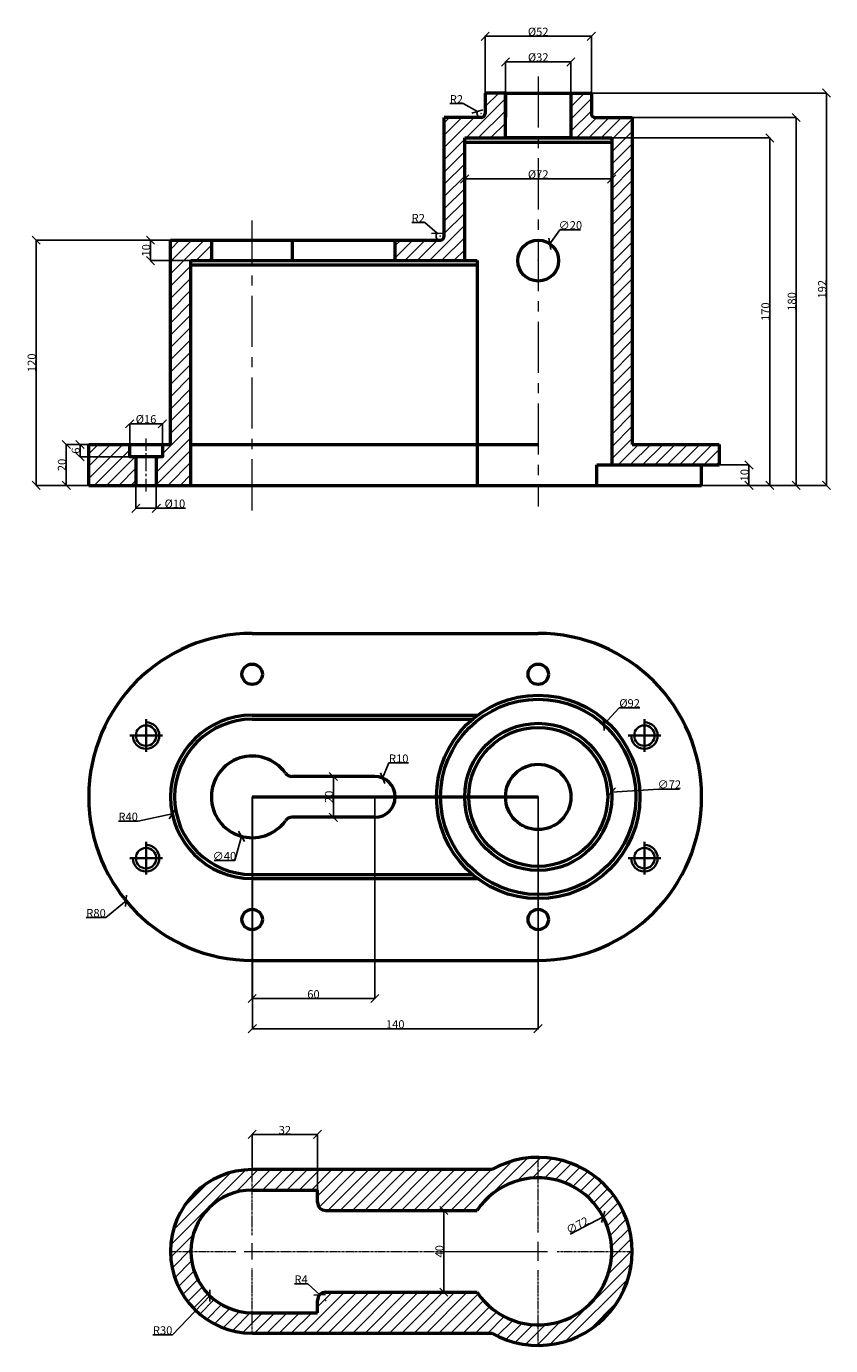
# Model space of a CAD drawing. Units: millimetres. Extents: x 219 to 612, y 65 to 711.
import ezdxf

# ---------------------------------------------------------------- set-up
doc = ezdxf.new("R2010")
doc.units = ezdxf.units.MM
doc.header["$MEASUREMENT"] = 0
doc.header["$PDMODE"] = 3
doc.header["$PDSIZE"] = -8
doc.linetypes.add('CENTER', pattern=[2, 1.25, -0.25, 0.25, -0.25])
for name, color, linetype, lineweight in [('M-CNTR', 1, 'CENTER', 18), ('M-DIMS', 2, 'Continuous', 25), ('M-FAST', 7, 'Continuous', 35), ('M-HATC', 8, 'Continuous', 18), ('M-OUTL', 7, 'Continuous', 50)]:
    doc.layers.add(name, color=color, linetype=linetype, lineweight=lineweight)
doc.styles.get("Standard").update_dxf_attribs({"font": 'arial.ttf'})
doc.dimstyles.get("Standard").update_dxf_attribs({"dimtxt": 4, "dimasz": 4, "dimexe": 0.18, "dimexo": 0.0625, "dimgap": 0.09, "dimtad": 1, "dimtoh": 1, "dimdec": 0, "dimzin": 0, "dimdsep": 46, "dimtxsty": 'Standard', "dimblk": 'OBLIQUE', "dimcen": 0.09, "dimclre": 251, "dimadec": 0, "dimazin": 0, "dimtfac": 1, "dimtdec": 0, "dimtofl": 0, "dimtmove": 0, "dimatfit": 3, "dimfxl": 1, "dimtolj": 1, "dimtzin": 0, "dimarcsym": 0})

# ---------------------------------------------------------------- blocks, each defined once
blk = doc.blocks.new('_Oblique')
at = {"color": 0, "linetype": 'ByBlock', "lineweight": -2}
blk.add_line((-0.5, -0.5), (0.5, 0.5), dxfattribs=at)
blk = doc.blocks.new('*D2')
at = {"layer": 'Defpoints', "color": 0, "transparency": 16777216}
for p in [(505.08, 336.11), (433.23, 331.42)]:
    blk.add_point(p, dxfattribs=at)
at = {"layer": 'M-DIMS', "color": 0, "lineweight": -2, "transparency": 16777216}
for p, q in [((528.23, 337.62), (505.08, 336.11)), ((538.36, 337.62), (528.23, 337.62)), ((469.07, 333.77), (469.25, 333.77)), ((469.16, 333.68), (469.16, 333.86))]:
    blk.add_line(p, q, dxfattribs=at)
at = {"layer": 'M-DIMS', "color": 0, "lineweight": -2, "transparency": 16777216, "xscale": 4, "yscale": 4, "zscale": 4, "rotation": 183.7310328163997}
blk.add_blockref('_Oblique', (505.08, 336.11), dxfattribs=at)
at = {"layer": 'M-DIMS', "color": 0, "transparency": 16777216, "insert": (533.34, 339.86), "char_height": 4, "attachment_point": 5}
blk.add_mtext('\\A1;∅72', dxfattribs=at)
blk = doc.blocks.new('*D3')
at = {"layer": 'Defpoints', "color": 0, "transparency": 16777216}
for p in [(495.16, 705.94), (443.16, 678.2), (495.16, 678.2)]:
    blk.add_point(p, dxfattribs=at)
at = {"layer": 'M-DIMS', "color": 0, "lineweight": -2, "transparency": 16777216}
for p, q in [((443.16, 678.27), (443.16, 706.12)), ((443.16, 705.94), (495.16, 705.94)), ((495.16, 678.27), (495.16, 706.12))]:
    blk.add_line(p, q, dxfattribs=at)
at = {"layer": 'M-DIMS', "color": 0, "lineweight": -2, "transparency": 16777216, "xscale": 4, "yscale": 4, "zscale": 4, "rotation": 180}
blk.add_blockref('_Oblique', (443.16, 705.94), dxfattribs=at)
at = {"layer": 'M-DIMS', "color": 0, "lineweight": -2, "transparency": 16777216, "xscale": 4, "yscale": 4, "zscale": 4}
blk.add_blockref('_Oblique', (495.16, 705.94), dxfattribs=at)
at = {"layer": 'M-DIMS', "color": 0, "transparency": 16777216, "insert": (469.16, 708.18), "char_height": 4, "attachment_point": 5}
blk.add_mtext('\\A1;%%C52', dxfattribs=at)
blk = doc.blocks.new('*D4')
at = {"layer": 'Defpoints', "color": 0, "transparency": 16777216}
for p in [(485.16, 693.41), (453.16, 678.2), (485.16, 678.2)]:
    blk.add_point(p, dxfattribs=at)
at = {"layer": 'M-DIMS', "color": 0, "lineweight": -2, "transparency": 16777216}
for p, q in [((453.16, 678.27), (453.16, 693.59)), ((453.16, 693.41), (485.16, 693.41)), ((485.16, 678.27), (485.16, 693.59))]:
    blk.add_line(p, q, dxfattribs=at)
at = {"layer": 'M-DIMS', "color": 0, "lineweight": -2, "transparency": 16777216, "xscale": 4, "yscale": 4, "zscale": 4, "rotation": 180}
blk.add_blockref('_Oblique', (453.16, 693.41), dxfattribs=at)
at = {"layer": 'M-DIMS', "color": 0, "lineweight": -2, "transparency": 16777216, "xscale": 4, "yscale": 4, "zscale": 4}
blk.add_blockref('_Oblique', (485.16, 693.41), dxfattribs=at)
at = {"layer": 'M-DIMS', "color": 0, "transparency": 16777216, "insert": (469.16, 695.65), "char_height": 4, "attachment_point": 5}
blk.add_mtext('\\A1;%%C32', dxfattribs=at)
blk = doc.blocks.new('*D5')
at = {"layer": 'Defpoints', "color": 0, "transparency": 16777216}
for p in [(549.16, 496.2), (572.3, 496.2), (549.16, 486.2)]:
    blk.add_point(p, dxfattribs=at)
at = {"layer": 'M-DIMS', "color": 0, "lineweight": -2, "transparency": 16777216}
for p, q in [((549.22, 496.2), (572.48, 496.2)), ((572.3, 486.2), (572.3, 496.2)), ((549.22, 486.2), (572.48, 486.2))]:
    blk.add_line(p, q, dxfattribs=at)
at = {"layer": 'M-DIMS', "color": 0, "lineweight": -2, "transparency": 16777216, "xscale": 4, "yscale": 4, "zscale": 4}
for p, rotation in [((572.3, 496.2), 90), ((572.3, 486.2), 270)]:
    blk.add_blockref('_Oblique', p, dxfattribs=dict(at, rotation=rotation))
at = {"layer": 'M-DIMS', "color": 0, "transparency": 16777216, "insert": (570.17, 491.2), "char_height": 4, "attachment_point": 5, "rotation": 90}
blk.add_mtext('\\A1;10', dxfattribs=at)
blk = doc.blocks.new('*D6')
at = {"layer": 'Defpoints', "color": 0, "transparency": 16777216}
for p in [(505.13, 656.2), (582.55, 656.2), (549.16, 486.2)]:
    blk.add_point(p, dxfattribs=at)
at = {"layer": 'M-DIMS', "color": 0, "lineweight": -2, "transparency": 16777216}
for p, q in [((505.2, 656.2), (582.73, 656.2)), ((582.55, 486.2), (582.55, 656.2)), ((549.22, 486.2), (582.73, 486.2))]:
    blk.add_line(p, q, dxfattribs=at)
at = {"layer": 'M-DIMS', "color": 0, "lineweight": -2, "transparency": 16777216, "xscale": 4, "yscale": 4, "zscale": 4}
for p, rotation in [((582.55, 656.2), 90), ((582.55, 486.2), 270)]:
    blk.add_blockref('_Oblique', p, dxfattribs=dict(at, rotation=rotation))
at = {"layer": 'M-DIMS', "color": 0, "transparency": 16777216, "insert": (580.42, 571.2), "char_height": 4, "attachment_point": 5, "rotation": 90}
blk.add_mtext('\\A1;170', dxfattribs=at)
blk = doc.blocks.new('*D7')
at = {"layer": 'Defpoints', "color": 0, "transparency": 16777216}
for p in [(515.13, 666.2), (595.44, 666.2), (549.16, 486.2)]:
    blk.add_point(p, dxfattribs=at)
at = {"layer": 'M-DIMS', "color": 0, "lineweight": -2, "transparency": 16777216}
for p, q in [((515.2, 666.2), (595.62, 666.2)), ((595.44, 486.2), (595.44, 666.2)), ((549.22, 486.2), (595.62, 486.2))]:
    blk.add_line(p, q, dxfattribs=at)
at = {"layer": 'M-DIMS', "color": 0, "lineweight": -2, "transparency": 16777216, "xscale": 4, "yscale": 4, "zscale": 4}
for p, rotation in [((595.44, 666.2), 90), ((595.44, 486.2), 270)]:
    blk.add_blockref('_Oblique', p, dxfattribs=dict(at, rotation=rotation))
at = {"layer": 'M-DIMS', "color": 0, "transparency": 16777216, "insert": (593.31, 576.2), "char_height": 4, "attachment_point": 5, "rotation": 90}
blk.add_mtext('\\A1;180', dxfattribs=at)
blk = doc.blocks.new('*D8')
at = {"layer": 'Defpoints', "color": 0, "transparency": 16777216}
for p in [(495.16, 678.2), (610.29, 678.2), (549.16, 486.2)]:
    blk.add_point(p, dxfattribs=at)
at = {"layer": 'M-DIMS', "color": 0, "lineweight": -2, "transparency": 16777216}
for p, q in [((495.22, 678.2), (610.47, 678.2)), ((610.29, 486.2), (610.29, 678.2)), ((549.22, 486.2), (610.47, 486.2))]:
    blk.add_line(p, q, dxfattribs=at)
at = {"layer": 'M-DIMS', "color": 0, "lineweight": -2, "transparency": 16777216, "xscale": 4, "yscale": 4, "zscale": 4}
for p, rotation in [((610.29, 678.2), 90), ((610.29, 486.2), 270)]:
    blk.add_blockref('_Oblique', p, dxfattribs=dict(at, rotation=rotation))
at = {"layer": 'M-DIMS', "color": 0, "transparency": 16777216, "insert": (608.15, 582.2), "char_height": 4, "attachment_point": 5, "rotation": 90}
blk.add_mtext('\\A1;192', dxfattribs=at)
blk = doc.blocks.new('*D9')
at = {"layer": 'Defpoints', "color": 0, "transparency": 16777216}
for p in [(433.16, 641.83), (505.13, 641.83), (505.13, 636.16)]:
    blk.add_point(p, dxfattribs=at)
at = {"layer": 'M-DIMS', "color": 0, "lineweight": -2, "transparency": 16777216}
for p, q in [((433.16, 641.76), (433.16, 635.98)), ((505.13, 641.76), (505.13, 635.98)), ((433.16, 636.16), (505.13, 636.16))]:
    blk.add_line(p, q, dxfattribs=at)
at = {"layer": 'M-DIMS', "color": 0, "lineweight": -2, "transparency": 16777216, "xscale": 4, "yscale": 4, "zscale": 4, "rotation": 180}
blk.add_blockref('_Oblique', (433.16, 636.16), dxfattribs=at)
at = {"layer": 'M-DIMS', "color": 0, "lineweight": -2, "transparency": 16777216, "xscale": 4, "yscale": 4, "zscale": 4}
blk.add_blockref('_Oblique', (505.13, 636.16), dxfattribs=at)
at = {"layer": 'M-DIMS', "color": 0, "transparency": 16777216, "insert": (469.15, 638.4), "char_height": 4, "attachment_point": 5}
blk.add_mtext('\\A1;%%C72', dxfattribs=at)
blk = doc.blocks.new('*D10')
at = {"layer": 'Defpoints', "color": 0, "transparency": 16777216}
for p in [(289.16, 606.2), (279.37, 596.2), (299.16, 596.2)]:
    blk.add_point(p, dxfattribs=at)
at = {"layer": 'M-DIMS', "color": 0, "lineweight": -2, "transparency": 16777216}
for p, q in [((289.1, 606.2), (279.19, 606.2)), ((279.37, 606.2), (279.37, 596.2)), ((299.1, 596.2), (279.19, 596.2))]:
    blk.add_line(p, q, dxfattribs=at)
at = {"layer": 'M-DIMS', "color": 0, "lineweight": -2, "transparency": 16777216, "xscale": 4, "yscale": 4, "zscale": 4}
for p, rotation in [((279.37, 606.2), 90), ((279.37, 596.2), 270)]:
    blk.add_blockref('_Oblique', p, dxfattribs=dict(at, rotation=rotation))
at = {"layer": 'M-DIMS', "color": 0, "transparency": 16777216, "insert": (277.23, 601.2), "char_height": 4, "attachment_point": 5, "rotation": 90}
blk.add_mtext('\\A1;10', dxfattribs=at)
blk = doc.blocks.new('*D11')
at = {"layer": 'Defpoints', "color": 0, "transparency": 16777216}
for p in [(249.16, 506.2), (238.15, 486.2), (249.16, 486.2)]:
    blk.add_point(p, dxfattribs=at)
at = {"layer": 'M-DIMS', "color": 0, "lineweight": -2, "transparency": 16777216}
for p, q in [((249.1, 506.2), (237.97, 506.2)), ((238.15, 506.2), (238.15, 486.2)), ((249.1, 486.2), (237.97, 486.2))]:
    blk.add_line(p, q, dxfattribs=at)
at = {"layer": 'M-DIMS', "color": 0, "lineweight": -2, "transparency": 16777216, "xscale": 4, "yscale": 4, "zscale": 4}
for p, rotation in [((238.15, 506.2), 90), ((238.15, 486.2), 270)]:
    blk.add_blockref('_Oblique', p, dxfattribs=dict(at, rotation=rotation))
at = {"layer": 'M-DIMS', "color": 0, "transparency": 16777216, "insert": (236.02, 496.2), "char_height": 4, "attachment_point": 5, "rotation": 90}
blk.add_mtext('\\A1;20', dxfattribs=at)
blk = doc.blocks.new('*D12')
at = {"layer": 'Defpoints', "color": 0, "transparency": 16777216}
for p in [(223.39, 606.2), (289.16, 606.2), (249.16, 486.2)]:
    blk.add_point(p, dxfattribs=at)
at = {"layer": 'M-DIMS', "color": 0, "lineweight": -2, "transparency": 16777216}
for p, q in [((289.1, 606.2), (223.21, 606.2)), ((223.39, 486.2), (223.39, 606.2)), ((249.1, 486.2), (223.21, 486.2))]:
    blk.add_line(p, q, dxfattribs=at)
at = {"layer": 'M-DIMS', "color": 0, "lineweight": -2, "transparency": 16777216, "xscale": 4, "yscale": 4, "zscale": 4}
for p, rotation in [((223.39, 606.2), 90), ((223.39, 486.2), 270)]:
    blk.add_blockref('_Oblique', p, dxfattribs=dict(at, rotation=rotation))
at = {"layer": 'M-DIMS', "color": 0, "transparency": 16777216, "insert": (221.25, 546.2), "char_height": 4, "attachment_point": 5, "rotation": 90}
blk.add_mtext('\\A1;120', dxfattribs=at)
blk = doc.blocks.new('*D13')
at = {"layer": 'Defpoints', "color": 0, "transparency": 16777216}
for p in [(419.68, 609.54), (421.16, 608.2)]:
    blk.add_point(p, dxfattribs=at)
at = {"layer": 'M-DIMS', "color": 0, "lineweight": -2, "transparency": 16777216}
for p, q in [((407.25, 614.91), (413.74, 614.91)), ((413.74, 614.91), (419.68, 609.54)), ((421.07, 608.2), (421.25, 608.2)), ((421.16, 608.11), (421.16, 608.29))]:
    blk.add_line(p, q, dxfattribs=at)
blk.add_arc((421.16, 608.2), 2, 132.6877, 268.20951, dxfattribs=at)
at = {"layer": 'M-DIMS', "color": 0, "lineweight": -2, "transparency": 16777216, "xscale": 4, "yscale": 4, "zscale": 4, "rotation": 317.8443171203354}
blk.add_blockref('_Oblique', (419.68, 609.54), dxfattribs=at)
at = {"layer": 'M-DIMS', "color": 0, "transparency": 16777216, "insert": (410.45, 617.01), "char_height": 4, "attachment_point": 5}
blk.add_mtext('\\A1;R2', dxfattribs=at)
blk = doc.blocks.new('*D14')
at = {"layer": 'Defpoints', "color": 0, "transparency": 16777216}
for p in [(439.41, 669.18), (441.16, 668.2)]:
    blk.add_point(p, dxfattribs=at)
at = {"layer": 'M-DIMS', "color": 0, "lineweight": -2, "transparency": 16777216}
for p, q in [((425.92, 673.07), (432.42, 673.07)), ((432.42, 673.07), (439.41, 669.18)), ((441.07, 668.2), (441.25, 668.2)), ((441.16, 668.11), (441.16, 668.29))]:
    blk.add_line(p, q, dxfattribs=at)
blk.add_arc((441.16, 668.2), 2, 145.73791, 268.20951, dxfattribs=at)
at = {"layer": 'M-DIMS', "color": 0, "lineweight": -2, "transparency": 16777216, "xscale": 4, "yscale": 4, "zscale": 4, "rotation": 330.8945315013513}
blk.add_blockref('_Oblique', (439.41, 669.18), dxfattribs=at)
at = {"layer": 'M-DIMS', "color": 0, "transparency": 16777216, "insert": (429.13, 675.16), "char_height": 4, "attachment_point": 5}
blk.add_mtext('\\A1;R2', dxfattribs=at)
blk = doc.blocks.new('*D15')
at = {"layer": 'Defpoints', "color": 0, "transparency": 16777216}
for p in [(474.92, 604.38), (463.4, 588.03)]:
    blk.add_point(p, dxfattribs=at)
at = {"layer": 'M-DIMS', "color": 0, "lineweight": -2, "transparency": 16777216}
for p, q in [((479.77, 611.25), (474.92, 604.38)), ((489.93, 611.25), (479.77, 611.25)), ((469.07, 596.2), (469.25, 596.2)), ((469.16, 596.11), (469.16, 596.29))]:
    blk.add_line(p, q, dxfattribs=at)
at = {"layer": 'M-DIMS', "color": 0, "lineweight": -2, "transparency": 16777216, "xscale": 4, "yscale": 4, "zscale": 4, "rotation": 234.8190006468018}
blk.add_blockref('_Oblique', (474.92, 604.38), dxfattribs=at)
at = {"layer": 'M-DIMS', "color": 0, "transparency": 16777216, "insert": (484.89, 613.5), "char_height": 4, "attachment_point": 5}
blk.add_mtext('\\A1;∅20', dxfattribs=at)
blk = doc.blocks.new('*D16')
at = {"layer": 'Defpoints', "color": 0, "transparency": 16777216}
for p in [(285.2, 516.35), (269.2, 506.2), (285.2, 506.2)]:
    blk.add_point(p, dxfattribs=at)
at = {"layer": 'M-DIMS', "color": 0, "lineweight": -2, "transparency": 16777216}
for p, q in [((269.2, 506.27), (269.2, 516.53)), ((285.2, 506.27), (285.2, 516.53)), ((269.2, 516.35), (285.2, 516.35))]:
    blk.add_line(p, q, dxfattribs=at)
at = {"layer": 'M-DIMS', "color": 0, "lineweight": -2, "transparency": 16777216, "xscale": 4, "yscale": 4, "zscale": 4, "rotation": 180}
blk.add_blockref('_Oblique', (269.2, 516.35), dxfattribs=at)
at = {"layer": 'M-DIMS', "color": 0, "lineweight": -2, "transparency": 16777216, "xscale": 4, "yscale": 4, "zscale": 4}
blk.add_blockref('_Oblique', (285.2, 516.35), dxfattribs=at)
at = {"layer": 'M-DIMS', "color": 0, "transparency": 16777216, "insert": (277.2, 518.59), "char_height": 4, "attachment_point": 5}
blk.add_mtext('\\A1;%%C16', dxfattribs=at)
blk = doc.blocks.new('*D17')
at = {"layer": 'Defpoints', "color": 0, "transparency": 16777216}
for p in [(244.91, 506.2), (269.2, 506.2), (269.2, 500.2)]:
    blk.add_point(p, dxfattribs=at)
at = {"layer": 'M-DIMS', "color": 0, "lineweight": -2, "transparency": 16777216}
for p, q in [((269.13, 506.2), (244.73, 506.2)), ((244.91, 500.2), (244.91, 506.2)), ((269.13, 500.2), (244.73, 500.2))]:
    blk.add_line(p, q, dxfattribs=at)
at = {"layer": 'M-DIMS', "color": 0, "lineweight": -2, "transparency": 16777216, "xscale": 4, "yscale": 4, "zscale": 4}
for p, rotation in [((244.91, 506.2), 90), ((244.91, 500.2), 270)]:
    blk.add_blockref('_Oblique', p, dxfattribs=dict(at, rotation=rotation))
at = {"layer": 'M-DIMS', "color": 0, "transparency": 16777216, "insert": (242.78, 503.2), "char_height": 4, "attachment_point": 5, "rotation": 90}
blk.add_mtext('\\A1;6', dxfattribs=at)
blk = doc.blocks.new('*D18')
at = {"layer": 'Defpoints', "color": 0, "transparency": 16777216}
for p in [(272.2, 486.2), (282.2, 486.2), (282.2, 475.01)]:
    blk.add_point(p, dxfattribs=at)
at = {"layer": 'M-DIMS', "color": 0, "lineweight": -2, "transparency": 16777216}
for p, q in [((272.2, 486.14), (272.2, 474.83)), ((282.2, 486.14), (282.2, 474.83)), ((272.2, 475.01), (282.2, 475.01)), ((282.2, 475.01), (296.44, 475.01))]:
    blk.add_line(p, q, dxfattribs=at)
at = {"layer": 'M-DIMS', "color": 0, "lineweight": -2, "transparency": 16777216, "xscale": 4, "yscale": 4, "zscale": 4, "rotation": 180}
blk.add_blockref('_Oblique', (272.2, 475.01), dxfattribs=at)
at = {"layer": 'M-DIMS', "color": 0, "lineweight": -2, "transparency": 16777216, "xscale": 4, "yscale": 4, "zscale": 4}
blk.add_blockref('_Oblique', (282.2, 475.01), dxfattribs=at)
at = {"layer": 'M-DIMS', "color": 0, "transparency": 16777216, "insert": (291.32, 477.26), "char_height": 4, "attachment_point": 5}
blk.add_mtext('\\A1;%%C10', dxfattribs=at)
blk = doc.blocks.new('*U19')
at = {"layer": 'M-CNTR', "color": 0, "transparency": 16777216}
for p, q in [((0, 8), (0, 40.12)), ((-40.12, 0), (-8, 0)), ((8, 0), (40.12, 0)), ((0, -40.12), (0, -8))]:
    blk.add_line(p, q, dxfattribs=at)
at = {"layer": 'M-CNTR', "color": 0, "linetype": 'Continuous', "transparency": 16777216}
for p, q in [((-4, 0), (4, 0)), ((0, -4), (0, 4))]:
    blk.add_line(p, q, dxfattribs=at)
blk = doc.blocks.new('*U20')
at = {"layer": 'M-CNTR', "color": 0, "transparency": 16777216}
for p, q in [((0, 9.2), (0, 46.12)), ((-46.12, 0), (-9.2, 0)), ((9.2, 0), (46.12, 0)), ((0, -46.12), (0, -9.2))]:
    blk.add_line(p, q, dxfattribs=at)
at = {"layer": 'M-CNTR', "color": 0, "linetype": 'Continuous', "transparency": 16777216}
for p, q in [((-4.6, 0), (4.6, 0)), ((0, -4.6), (0, 4.6))]:
    blk.add_line(p, q, dxfattribs=at)
blk = doc.blocks.new('*D21')
at = {"layer": 'Defpoints', "color": 0, "transparency": 16777216}
for p in [(329.16, 111.38), (308.44, 89.69)]:
    blk.add_point(p, dxfattribs=at)
at = {"layer": 'M-DIMS', "color": 0, "lineweight": -2, "transparency": 16777216}
for p, q in [((329.07, 111.38), (329.25, 111.38)), ((329.16, 111.29), (329.16, 111.47)), ((290.2, 70.59), (308.44, 89.69)), ((280.56, 70.59), (290.2, 70.59))]:
    blk.add_line(p, q, dxfattribs=at)
at = {"layer": 'M-DIMS', "color": 0, "lineweight": -2, "transparency": 16777216, "xscale": 4, "yscale": 4, "zscale": 4, "rotation": 46.31825092677839}
blk.add_blockref('_Oblique', (308.44, 89.69), dxfattribs=at)
at = {"layer": 'M-DIMS', "color": 0, "transparency": 16777216, "insert": (285.33, 72.72), "char_height": 4, "attachment_point": 5}
blk.add_mtext('\\A1;R30', dxfattribs=at)
blk = doc.blocks.new('*D22')
at = {"layer": 'Defpoints', "color": 0, "transparency": 16777216}
for p in [(362.23, 90.11), (365.16, 87.38)]:
    blk.add_point(p, dxfattribs=at)
at = {"layer": 'M-DIMS', "color": 0, "lineweight": -2, "transparency": 16777216}
for p, q in [((349.86, 95.57), (356.39, 95.57)), ((356.39, 95.57), (362.23, 90.11)), ((365.07, 87.38), (365.25, 87.38)), ((365.16, 87.29), (365.16, 87.47))]:
    blk.add_line(p, q, dxfattribs=at)
at = {"layer": 'M-DIMS', "color": 0, "lineweight": -2, "transparency": 16777216, "xscale": 4, "yscale": 4, "zscale": 4, "rotation": 316.9612677610523}
blk.add_blockref('_Oblique', (362.23, 90.11), dxfattribs=at)
at = {"layer": 'M-DIMS', "color": 0, "transparency": 16777216, "insert": (353.08, 97.66), "char_height": 4, "attachment_point": 5}
blk.add_mtext('\\A1;R4', dxfattribs=at)
blk = doc.blocks.new('*D23')
at = {"layer": 'Defpoints', "color": 0, "transparency": 16777216}
for p in [(361.16, 168.61), (329.16, 151.38), (361.16, 141.38)]:
    blk.add_point(p, dxfattribs=at)
at = {"layer": 'M-DIMS', "color": 0, "lineweight": -2, "transparency": 16777216}
for p, q in [((329.16, 151.44), (329.16, 168.79)), ((329.16, 168.61), (361.16, 168.61)), ((361.16, 141.44), (361.16, 168.79))]:
    blk.add_line(p, q, dxfattribs=at)
at = {"layer": 'M-DIMS', "color": 0, "lineweight": -2, "transparency": 16777216, "xscale": 4, "yscale": 4, "zscale": 4, "rotation": 180}
blk.add_blockref('_Oblique', (329.16, 168.61), dxfattribs=at)
at = {"layer": 'M-DIMS', "color": 0, "lineweight": -2, "transparency": 16777216, "xscale": 4, "yscale": 4, "zscale": 4}
blk.add_blockref('_Oblique', (361.16, 168.61), dxfattribs=at)
at = {"layer": 'M-DIMS', "color": 0, "transparency": 16777216, "insert": (345.16, 170.74), "char_height": 4, "attachment_point": 5}
blk.add_mtext('\\A1;32', dxfattribs=at)
blk = doc.blocks.new('*D24')
at = {"layer": 'Defpoints', "color": 0, "transparency": 16777216}
for p in [(422.97, 131.38), (422.97, 91.38), (422.97, 91.38)]:
    blk.add_point(p, dxfattribs=at)
at = {"layer": 'M-DIMS', "color": 0, "lineweight": -2, "transparency": 16777216}
for p, q in [((422.97, 131.38), (422.97, 91.38)), ((423.03, 131.38), (423.15, 131.38)), ((423.03, 91.38), (423.15, 91.38))]:
    blk.add_line(p, q, dxfattribs=at)
at = {"layer": 'M-DIMS', "color": 0, "lineweight": -2, "transparency": 16777216, "xscale": 4, "yscale": 4, "zscale": 4}
for p, rotation in [((422.97, 131.38), 90), ((422.97, 91.38), 270)]:
    blk.add_blockref('_Oblique', p, dxfattribs=dict(at, rotation=rotation))
at = {"layer": 'M-DIMS', "color": 0, "transparency": 16777216, "insert": (420.84, 111.38), "char_height": 4, "attachment_point": 5, "rotation": 90}
blk.add_mtext('\\A1;40', dxfattribs=at)
blk = doc.blocks.new('*D25')
at = {"layer": 'Defpoints', "color": 0, "transparency": 16777216}
for p in [(500.95, 128.28), (437.37, 94.49)]:
    blk.add_point(p, dxfattribs=at)
at = {"layer": 'M-DIMS', "color": 0, "lineweight": -2, "transparency": 16777216}
blk.add_line((484.86, 119.73), (500.95, 128.28), dxfattribs=at)
at = {"layer": 'M-DIMS', "color": 0, "lineweight": -2, "transparency": 16777216, "xscale": 4, "yscale": 4, "zscale": 4, "rotation": 27.98972958099295}
blk.add_blockref('_Oblique', (500.95, 128.28), dxfattribs=at)
at = {"layer": 'M-DIMS', "color": 0, "transparency": 16777216, "insert": (488.32, 124.11), "char_height": 4, "attachment_point": 5, "rotation": 27.98973}
blk.add_mtext('\\A1;∅72', dxfattribs=at)
blk = doc.blocks.new('*D26')
at = {"layer": 'Defpoints', "color": 0, "transparency": 16777216}
for p in [(329.16, 333.77), (290.03, 325.47)]:
    blk.add_point(p, dxfattribs=at)
at = {"layer": 'M-DIMS', "color": 0, "lineweight": -2, "transparency": 16777216}
for p, q in [((329.07, 333.77), (329.25, 333.77)), ((329.16, 333.68), (329.16, 333.86)), ((273.29, 321.92), (290.03, 325.47)), ((263.66, 321.92), (273.29, 321.92))]:
    blk.add_line(p, q, dxfattribs=at)
at = {"layer": 'M-DIMS', "color": 0, "lineweight": -2, "transparency": 16777216, "xscale": 4, "yscale": 4, "zscale": 4, "rotation": 11.97301703916849}
blk.add_blockref('_Oblique', (290.03, 325.47), dxfattribs=at)
at = {"layer": 'M-DIMS', "color": 0, "transparency": 16777216, "insert": (268.43, 324.05), "char_height": 4, "attachment_point": 5}
blk.add_mtext('\\A1;R40', dxfattribs=at)
blk = doc.blocks.new('*D27')
at = {"layer": 'Defpoints', "color": 0, "transparency": 16777216}
for p in [(329.16, 333.77), (267.42, 282.88)]:
    blk.add_point(p, dxfattribs=at)
at = {"layer": 'M-DIMS', "color": 0, "lineweight": -2, "transparency": 16777216}
for p, q in [((329.07, 333.77), (329.25, 333.77)), ((329.16, 333.68), (329.16, 333.86)), ((257.59, 274.78), (267.42, 282.88)), ((247.95, 274.78), (257.59, 274.78))]:
    blk.add_line(p, q, dxfattribs=at)
at = {"layer": 'M-DIMS', "color": 0, "lineweight": -2, "transparency": 16777216, "xscale": 4, "yscale": 4, "zscale": 4, "rotation": 39.49456413514449}
blk.add_blockref('_Oblique', (267.42, 282.88), dxfattribs=at)
at = {"layer": 'M-DIMS', "color": 0, "transparency": 16777216, "insert": (252.73, 276.91), "char_height": 4, "attachment_point": 5}
blk.add_mtext('\\A1;R80', dxfattribs=at)
blk = doc.blocks.new('*D28')
at = {"layer": 'Defpoints', "color": 0, "transparency": 16777216}
for p in [(501.31, 369.13), (437.01, 298.4)]:
    blk.add_point(p, dxfattribs=at)
at = {"layer": 'M-DIMS', "color": 0, "lineweight": -2, "transparency": 16777216}
for p, q in [((508.76, 377.33), (501.31, 369.13)), ((518.91, 377.33), (508.76, 377.33)), ((469.07, 333.77), (469.25, 333.77)), ((469.16, 333.68), (469.16, 333.86))]:
    blk.add_line(p, q, dxfattribs=at)
at = {"layer": 'M-DIMS', "color": 0, "lineweight": -2, "transparency": 16777216, "xscale": 4, "yscale": 4, "zscale": 4, "rotation": 227.7279978336799}
blk.add_blockref('_Oblique', (501.31, 369.13), dxfattribs=at)
at = {"layer": 'M-DIMS', "color": 0, "transparency": 16777216, "insert": (513.89, 379.58), "char_height": 4, "width": 10.0791, "attachment_point": 5}
blk.add_mtext('\\A1;%%C92', dxfattribs=at)
blk = doc.blocks.new('*D29')
at = {"layer": 'Defpoints', "color": 0, "transparency": 16777216}
for p in [(329.16, 333.68), (389.16, 333.77), (389.16, 235.08)]:
    blk.add_point(p, dxfattribs=at)
at = {"layer": 'M-DIMS', "color": 0, "lineweight": -2, "transparency": 16777216}
for p, q in [((329.16, 333.61), (329.16, 234.9)), ((389.16, 333.7), (389.16, 234.9)), ((329.16, 235.08), (389.16, 235.08))]:
    blk.add_line(p, q, dxfattribs=at)
at = {"layer": 'M-DIMS', "color": 0, "lineweight": -2, "transparency": 16777216, "xscale": 4, "yscale": 4, "zscale": 4, "rotation": 180}
blk.add_blockref('_Oblique', (329.16, 235.08), dxfattribs=at)
at = {"layer": 'M-DIMS', "color": 0, "lineweight": -2, "transparency": 16777216, "xscale": 4, "yscale": 4, "zscale": 4}
blk.add_blockref('_Oblique', (389.16, 235.08), dxfattribs=at)
at = {"layer": 'M-DIMS', "color": 0, "transparency": 16777216, "insert": (359.16, 237.21), "char_height": 4, "attachment_point": 5}
blk.add_mtext('\\A1;60', dxfattribs=at)
blk = doc.blocks.new('*D30')
at = {"layer": 'Defpoints', "color": 0, "transparency": 16777216}
for p in [(329.25, 333.77), (469.07, 333.77), (469.07, 220.35)]:
    blk.add_point(p, dxfattribs=at)
at = {"layer": 'M-DIMS', "color": 0, "lineweight": -2, "transparency": 16777216}
for p, q in [((329.25, 333.7), (329.25, 220.17)), ((469.07, 333.7), (469.07, 220.17)), ((329.25, 220.35), (469.07, 220.35))]:
    blk.add_line(p, q, dxfattribs=at)
at = {"layer": 'M-DIMS', "color": 0, "lineweight": -2, "transparency": 16777216, "xscale": 4, "yscale": 4, "zscale": 4, "rotation": 180}
blk.add_blockref('_Oblique', (329.25, 220.35), dxfattribs=at)
at = {"layer": 'M-DIMS', "color": 0, "lineweight": -2, "transparency": 16777216, "xscale": 4, "yscale": 4, "zscale": 4}
blk.add_blockref('_Oblique', (469.07, 220.35), dxfattribs=at)
at = {"layer": 'M-DIMS', "color": 0, "transparency": 16777216, "insert": (399.16, 222.48), "char_height": 4, "attachment_point": 5}
blk.add_mtext('\\A1;140', dxfattribs=at)
blk = doc.blocks.new('*D31')
at = {"layer": 'Defpoints', "color": 0, "transparency": 16777216}
for p in [(368.9, 343.77), (368.9, 343.77), (368.9, 323.77)]:
    blk.add_point(p, dxfattribs=at)
at = {"layer": 'M-DIMS', "color": 0, "lineweight": -2, "transparency": 16777216}
for p, q in [((368.9, 323.77), (368.9, 343.77)), ((368.97, 343.77), (369.08, 343.77)), ((368.97, 323.77), (369.08, 323.77))]:
    blk.add_line(p, q, dxfattribs=at)
at = {"layer": 'M-DIMS', "color": 0, "lineweight": -2, "transparency": 16777216, "xscale": 4, "yscale": 4, "zscale": 4}
for p, rotation in [((368.9, 343.77), 90), ((368.9, 323.77), 270)]:
    blk.add_blockref('_Oblique', p, dxfattribs=dict(at, rotation=rotation))
at = {"layer": 'M-DIMS', "color": 0, "transparency": 16777216, "insert": (366.77, 333.77), "char_height": 4, "attachment_point": 5, "rotation": 90}
blk.add_mtext('\\A1;20', dxfattribs=at)
blk = doc.blocks.new('*D32')
at = {"layer": 'Defpoints', "color": 0, "transparency": 16777216}
for p in [(334.41, 353.06), (323.91, 314.47)]:
    blk.add_point(p, dxfattribs=at)
at = {"layer": 'M-DIMS', "color": 0, "lineweight": -2, "transparency": 16777216}
for p, q in [((329.07, 333.77), (329.25, 333.77)), ((329.16, 333.68), (329.16, 333.86)), ((320.68, 302.59), (323.91, 314.47)), ((310.52, 302.59), (320.68, 302.59))]:
    blk.add_line(p, q, dxfattribs=at)
at = {"layer": 'M-DIMS', "color": 0, "lineweight": -2, "transparency": 16777216, "xscale": 4, "yscale": 4, "zscale": 4, "rotation": 74.78872029744083}
blk.add_blockref('_Oblique', (323.91, 314.47), dxfattribs=at)
at = {"layer": 'M-DIMS', "color": 0, "transparency": 16777216, "insert": (315.56, 304.83), "char_height": 4, "attachment_point": 5}
blk.add_mtext('\\A1;∅40', dxfattribs=at)
blk = doc.blocks.new('*D33')
at = {"layer": 'Defpoints', "color": 0, "transparency": 16777216}
for p in [(392.97, 343.01), (389.16, 333.77)]:
    blk.add_point(p, dxfattribs=at)
at = {"layer": 'M-DIMS', "color": 0, "lineweight": -2, "transparency": 16777216}
for p, q in [((396.02, 350.41), (392.97, 343.01)), ((405.66, 350.41), (396.02, 350.41)), ((389.07, 333.77), (389.25, 333.77)), ((389.16, 333.68), (389.16, 333.86))]:
    blk.add_line(p, q, dxfattribs=at)
at = {"layer": 'M-DIMS', "color": 0, "lineweight": -2, "transparency": 16777216, "xscale": 4, "yscale": 4, "zscale": 4, "rotation": 247.5859450756733}
blk.add_blockref('_Oblique', (392.97, 343.01), dxfattribs=at)
at = {"layer": 'M-DIMS', "color": 0, "transparency": 16777216, "insert": (400.88, 352.54), "char_height": 4, "attachment_point": 5}
blk.add_mtext('\\A1;R10', dxfattribs=at)
blk = doc.blocks.new('HOLE-TAPPED')
for p, q in [((277.2, 371.77), (277.2, 355.77)), ((269.2, 363.77), (285.2, 363.77))]:
    blk.add_line(p, q)
blk.add_circle((277.2, 363.77), 5)
blk.add_arc((277.2, 363.77), 6.49, 180, 90)

msp = doc.modelspace()

# ---------------------------------------------------------------- hatches: boundary and pattern name
at = {"layer": 'M-HATC'}
h = msp.add_hatch(dxfattribs=at)
h.set_pattern_fill('ANSI31', color=256, scale=34)
h.paths.add_polyline_path([(453.16, 678.2), (443.16, 678.2), (443.16, 666.2), (423.16, 666.2), (423.16, 606.2), (399.16, 606.2), (399.16, 596.2), (433.16, 596.2), (433.16, 656.2), (453.16, 656.2)])
h.paths.add_polyline_path([(505.13, 656.2), (505.13, 496.2), (549.16, 496.2), (557.81, 496.2), (557.81, 506.2), (515.13, 506.2), (515.13, 666.2), (495.16, 666.2), (495.16, 678.2), (485.16, 678.2), (485.16, 656.2)])
h = msp.add_hatch(dxfattribs=at)
h.set_pattern_fill('ANSI31', color=256, scale=34)
h.paths.add_polyline_path([(272.2, 486.2), (272.2, 500.2), (269.2, 500.2), (269.2, 506.2), (249.16, 506.2), (249.16, 486.2)])
h.paths.add_polyline_path([(299.16, 596.2), (309.16, 596.2), (309.16, 606.2), (289.16, 606.2), (289.16, 506.2), (285.2, 506.2), (285.2, 500.2), (282.2, 500.2), (282.2, 486.2), (299.16, 486.2)])
h = msp.add_hatch(dxfattribs=at)
h.set_pattern_fill('ANSI31', color=256, scale=34)
h.set_pattern_definition([(45, (0, -331.0266), (-3.005204, 3.005204), [])])
h.paths.add_polyline_path([(329.16, 151.38, 1), (329.16, 71.38), (446.44, 71.38, 1.717891), (446.44, 151.38)])
h.paths.add_polyline_path([(439.22, 131.38, -3.296663), (439.22, 91.38), (365.16, 91.38, 0.414214), (361.16, 87.38), (361.16, 81.38), (329.16, 81.38, -1), (329.16, 141.38), (361.16, 141.38), (361.16, 135.38, 0.414214), (365.16, 131.38)], flags=16)

# ---------------------------------------------------------------- linework, layer by layer
at = {"layer": 'M-CNTR', "ltscale": 20}
for p, q in [((469.16, 686.27), (469.16, 475.86)), ((329.16, 473.98), (329.16, 615.86))]:
    msp.add_line(p, q, dxfattribs=at)
at = {"layer": 'M-CNTR', "ltscale": 5}
msp.add_line((277.2, 483.18), (277.2, 509.22), dxfattribs=at)
at = {"layer": 'M-CNTR'}
msp.add_line((329.16, 111.38), (469.16, 111.38), dxfattribs=at)
at = {"layer": 'M-OUTL'}
for p, q in [((453.16, 678.2), (443.16, 678.2)), ((443.16, 678.2), (443.16, 668.2)), ((453.16, 678.2), (453.16, 666.2)), ((485.16, 678.2), (495.16, 678.2)), ((495.16, 678.2), (495.16, 668.2)), ((423.16, 608.2), (423.16, 666.2)), ((441.16, 666.2), (423.16, 666.2)), ((497.16, 666.2), (515.13, 666.2)), ((515.13, 666.2), (515.13, 506.2)), ((433.16, 596.2), (433.16, 656.2)), ((433.16, 656.2), (505.13, 656.2)), ((433.16, 654.2), (505.13, 654.2)), ((505.13, 656.2), (505.13, 496.2)), ((289.16, 606.2), (421.16, 606.2)), ((289.16, 506.2), (289.16, 606.2)), ((309.16, 606.2), (309.16, 596.2)), ((348.65, 606.2), (348.65, 596.2)), ((399.16, 596.2), (399.16, 606.2)), ((299.16, 596.2), (439.22, 596.2)), ((299.16, 486.2), (299.16, 596.2)), ((299.16, 594.2), (439.22, 594.2)), ((439.22, 596.2), (439.22, 486.2)), ((249.16, 486.2), (249.16, 506.2)), ((249.16, 506.2), (289.16, 506.2)), ((299.16, 506.2), (469.16, 506.2)), ((515.13, 506.2), (557.81, 506.2)), ((557.81, 506.2), (557.81, 496.2)), ((272.2, 500.2), (272.2, 486.2)), ((282.2, 500.2), (282.2, 486.2)), ((497.88, 486.2), (497.88, 496.2)), ((497.88, 496.2), (549.16, 496.2)), ((549.16, 486.2), (549.16, 496.2)), ((549.16, 496.2), (557.81, 496.2)), ((249.16, 486.2), (549.16, 486.2)), ((249.16, 486.2), (549.16, 486.2)), ((329.16, 413.77), (469.16, 413.77)), ((329.16, 373.77), (439.5, 373.77)), ((329.16, 371.77), (436.98, 371.77)), ((389.16, 343.77), (348.65, 343.77)), ((329.16, 333.77), (469.16, 333.77)), ((389.16, 323.77), (348.65, 323.77)), ((329.16, 295.77), (436.98, 295.77)), ((329.16, 293.77), (439.5, 293.77)), ((329.16, 253.77), (469.16, 253.77)), ((329.16, 141.38), (361.16, 141.38)), ((361.16, 135.38), (361.16, 141.38)), ((365.16, 131.38), (439.22, 131.38)), ((365.16, 91.38), (439.22, 91.38)), ((361.16, 81.38), (361.16, 87.38)), ((329.16, 81.38), (361.16, 81.38))]:
    msp.add_line(p, q, dxfattribs=at)
for points in [[(453.16, 678.2), (485.16, 678.2), (485.16, 656.2), (453.16, 656.2)], [(269.2, 506.2), (285.2, 506.2), (285.2, 500.2), (269.2, 500.2)]]:
    msp.add_lwpolyline(points, close=True, dxfattribs=at)
msp.add_lwpolyline([(446.44, 151.38), (329.16, 151.38, 1), (329.16, 71.38), (446.44, 71.38)], format="xyb", dxfattribs=at)
for centre, radius in [((469.16, 596.2), 10), ((329.16, 393.77), 5), ((469.16, 393.77), 5), ((469.16, 333.77), 49.79), ((469.16, 333.77), 47.79), ((469.16, 333.77), 36), ((469.16, 333.77), 34), ((469.16, 333.77), 16), ((329.16, 273.77), 5), ((469.16, 273.77), 5)]:
    msp.add_circle(centre, radius, dxfattribs=at)
for centre, radius, start, end in [((441.16, 668.2), 2, 270, 0), ((497.16, 668.2), 2, 180, 270), ((421.16, 608.2), 2, 270, 0), ((329.16, 333.77), 80, 90, 270), ((469.16, 333.77), 80, 270, 90), ((329.16, 333.77), 40, 90, 270), ((329.16, 333.77), 38, 90, 270), ((329.16, 333.77), 20, 35.68533, 324.31467), ((348.65, 347.77), 4, 215.68533, 270), ((389.16, 333.77), 10, 270, 90), ((348.65, 319.77), 4, 90, 144.31467), ((469.16, 111.38), 46, 240.40815, 119.59185), ((469.16, 111.38), 36, 213.74899, 146.25101), ((329.16, 111.38), 30, 90, 270), ((365.16, 135.38), 4, 180, 270), ((365.16, 87.38), 4, 90, 180)]:
    msp.add_arc(centre, radius, start, end, dxfattribs=at)

# ---------------------------------------------------------------- block references
at = {"layer": 'M-CNTR'}
for name, p in [('*U20', (469.16, 111.38)), ('*U19', (329.16, 111.38))]:
    msp.add_blockref(name, p, dxfattribs=at)
at = {"layer": 'M-FAST'}
for p in [(0, 0), (243.92, 0), (0, -60), (243.92, -60)]:
    msp.add_blockref('HOLE-TAPPED', p, dxfattribs=at)

# ---------------------------------------------------------------- dimensions: what is measured, and where the dimension line sits
at = {"layer": 'M-DIMS'}
for base, p1, p2, picture, middle in [((495.16, 705.94), (443.16, 678.2), (495.16, 678.2), '*D3', (469.16, 708.18)), ((485.16, 693.41), (453.16, 678.2), (485.16, 678.2), '*D4', (469.16, 695.65)), ((505.13, 636.16), (433.16, 641.83), (505.13, 641.83), '*D9', (469.15, 638.4)), ((285.2, 516.35), (269.2, 506.2), (285.2, 506.2), '*D16', (277.2, 518.59)), ((282.2, 475.01), (272.2, 486.2), (282.2, 486.2), '*D18', (291.32, 477.26))]:
    dim = msp.add_linear_dim(base=base, p1=p1, p2=p2, text='%%C<>', dimstyle='Standard', override={"dimclrd": 0, "dimclre": 0, "dimclrt": 0}, dxfattribs=at)
    dim.commit()
    dim.dimension.update_dxf_attribs({"geometry": picture, "text_midpoint": middle})
for base, p1, p2, picture, middle in [((610.29, 678.2), (549.16, 486.2), (495.16, 678.2), '*D8', (608.15, 582.2)), ((595.44, 666.2), (549.16, 486.2), (515.13, 666.2), '*D7', (593.31, 576.2)), ((582.55, 656.2), (549.16, 486.2), (505.13, 656.2), '*D6', (580.42, 571.2)), ((223.39, 606.2), (249.16, 486.2), (289.16, 606.2), '*D12', (221.25, 546.2)), ((279.37, 596.2), (289.16, 606.2), (299.16, 596.2), '*D10', (277.23, 601.2)), ((238.15, 486.2), (249.16, 506.2), (249.16, 486.2), '*D11', (236.02, 496.2)), ((244.91, 506.2), (269.2, 500.2), (269.2, 506.2), '*D17', (242.78, 503.2)), ((572.3, 496.2), (549.16, 486.2), (549.16, 496.2), '*D5', (570.17, 491.2)), ((368.9, 343.77), (368.9, 323.77), (368.9, 343.77), '*D31', (366.77, 333.77)), ((422.97, 91.38), (422.97, 131.38), (422.97, 91.38), '*D24', (420.84, 111.38))]:
    dim = msp.add_linear_dim(base=base, p1=p1, p2=p2, angle=90, dimstyle='Standard', override={"dimclrd": 0, "dimclre": 0, "dimclrt": 0}, dxfattribs=at)
    dim.commit()
    dim.dimension.update_dxf_attribs({"geometry": picture, "text_midpoint": middle})
for center, mpoint, picture, middle in [((441.16, 668.2), (439.41, 669.18), '*D14', (429.13, 675.16)), ((421.16, 608.2), (419.68, 609.54), '*D13', (410.45, 617.01)), ((389.16, 333.77), (392.97, 343.01), '*D33', (400.88, 352.54)), ((365.16, 87.38), (362.23, 90.11), '*D22', (353.08, 97.66))]:
    dim = msp.add_radius_dim(center=center, mpoint=mpoint, dimstyle='Standard', override={"dimclrd": 0, "dimclre": 0, "dimclrt": 0}, dxfattribs=at)
    dim.commit()
    dim.dimension.update_dxf_attribs({"geometry": picture, "text_midpoint": middle})
for p1, p2, picture, middle in [((463.4, 588.03), (474.92, 604.38), '*D15', (484.89, 611.25)), ((433.23, 331.42), (505.08, 336.11), '*D2', (528.23, 337.62)), ((437.37, 94.49), (500.95, 128.28), '*D25', (489.37, 122.12))]:
    dim = msp.add_diameter_dim_2p(p1=p1, p2=p2, dimstyle='Standard', override={"dimclrd": 0, "dimclre": 0, "dimclrt": 0}, dxfattribs=at)
    dim.commit()
    dim.dimension.update_dxf_attribs({"geometry": picture, "text_midpoint": middle, "dimtype": 163})
dim = msp.add_diameter_dim_2p(p1=(437.01, 298.4), p2=(501.31, 369.13), text='%%C92', dimstyle='Standard', override={"dimclrd": 0, "dimclre": 0, "dimclrt": 0}, dxfattribs=at)
dim.commit()
dim.dimension.update_dxf_attribs({"geometry": '*D28', "text_midpoint": (513.89, 377.33), "dimtype": 163})
dim = msp.add_diameter_dim_2p(p1=(334.41, 353.06), p2=(323.91, 314.47), dimstyle='Standard', override={"dimclrd": 0, "dimclre": 0, "dimclrt": 0}, dxfattribs=at)
dim.commit()
dim.dimension.update_dxf_attribs({"geometry": '*D32', "text_midpoint": (315.56, 304.83)})
for center, mpoint, picture, middle in [((329.16, 333.77), (267.42, 282.88), '*D27', (252.73, 274.78)), ((329.16, 333.77), (290.03, 325.47), '*D26', (273.29, 321.92)), ((329.16, 111.38), (308.44, 89.69), '*D21', (285.33, 70.59))]:
    dim = msp.add_radius_dim(center=center, mpoint=mpoint, dimstyle='Standard', override={"dimclrd": 0, "dimclre": 0, "dimclrt": 0}, dxfattribs=at)
    dim.commit()
    dim.dimension.update_dxf_attribs({"geometry": picture, "text_midpoint": middle, "dimtype": 164})
for base, p1, p2, picture, middle in [((389.16, 235.08), (329.16, 333.68), (389.16, 333.77), '*D29', (359.16, 237.21)), ((469.07, 220.35), (329.25, 333.77), (469.07, 333.77), '*D30', (399.16, 222.48)), ((361.16, 168.61), (329.16, 151.38), (361.16, 141.38), '*D23', (345.16, 170.74))]:
    dim = msp.add_linear_dim(base=base, p1=p1, p2=p2, dimstyle='Standard', override={"dimclrd": 0, "dimclre": 0, "dimclrt": 0}, dxfattribs=at)
    dim.commit()
    dim.dimension.update_dxf_attribs({"geometry": picture, "text_midpoint": middle})

doc.saveas('drawing.dxf')
